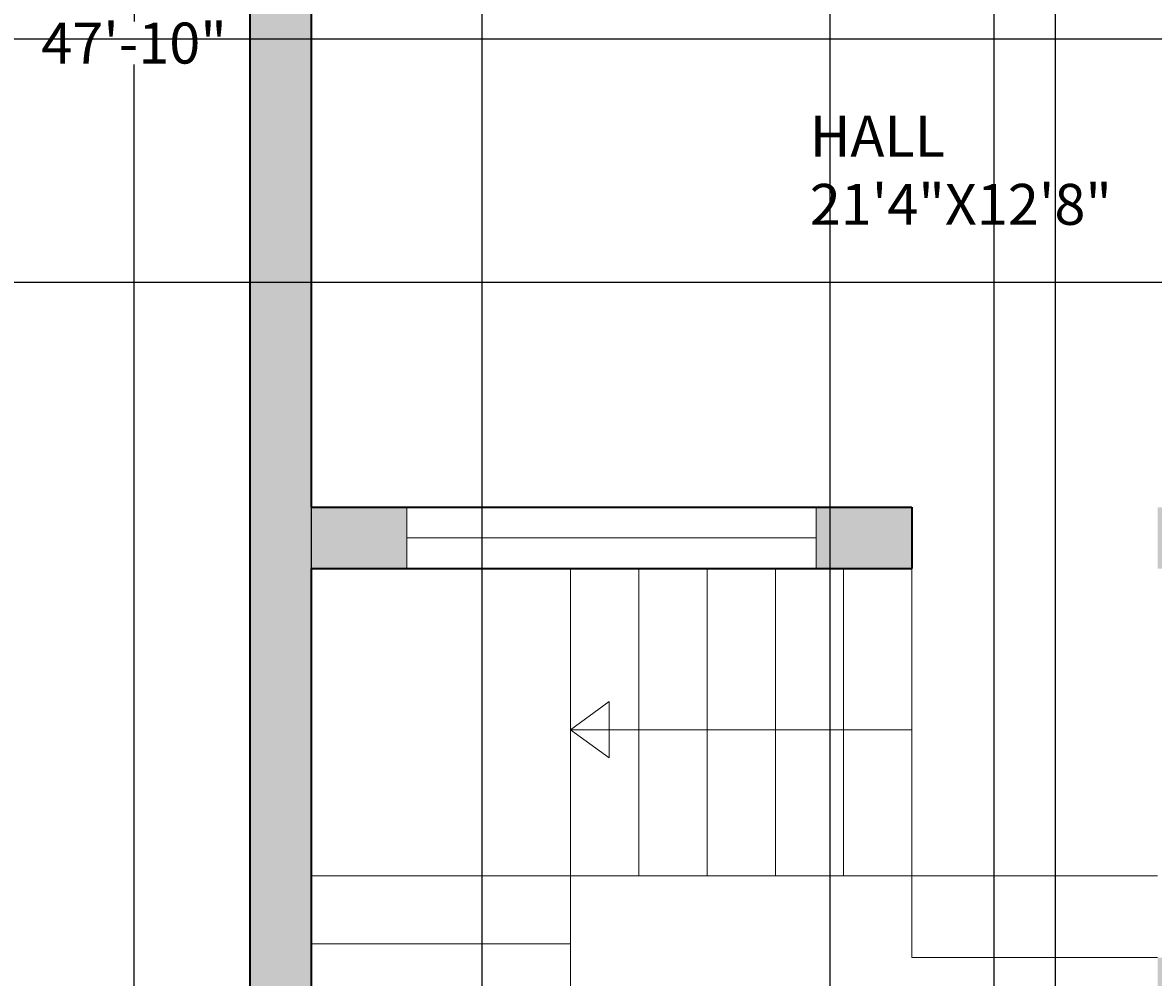
# Model space of a CAD drawing. Units: inches. Extents: x 37 to 706, y -568 to 110.
# Tile 15 of 24: x 361 to 526, y -373 to -233. Entities that reach past the tile are written whole.
import ezdxf

# ---------------------------------------------------------------- set-up
doc = ezdxf.new("R2010")
doc.units = ezdxf.units.IN
doc.header["$MEASUREMENT"] = 0
for name, color, linetype, lineweight in [('A-ANNO-DIMS', 2, 'Continuous', 18), ('A-AREA-IDEN', 7, 'Continuous', 18), ('A-FLOR-STRS', 7, 'Continuous', 18), ('A-GLAZ', 4, 'Continuous', 18), ('A-WALL', 7, 'Continuous', 35), ('A-WALL-PATT', 252, 'Continuous', 13)]:
    doc.layers.add(name, color=color, linetype=linetype, lineweight=lineweight)
doc.styles.get("Standard").update_dxf_attribs({"font": 'arial.ttf'})
doc.dimstyles.get("Standard").update_dxf_attribs({"dimtxt": 0.18, "dimasz": 0.18, "dimexe": 0.18, "dimexo": 0.0625, "dimgap": 0.09, "dimtad": 0, "dimtih": 1, "dimtoh": 1, "dimdec": 0, "dimzin": 0, "dimdsep": 46, "dimlunit": 3, "dimtxsty": 'Standard', "dimcen": 0.09, "dimadec": 0, "dimazin": 0, "dimtfac": 1, "dimtdec": 0, "dimtofl": 0, "dimtmove": 0, "dimatfit": 3, "dimfxl": 1, "dimtolj": 1, "dimtzin": 0, "dimarcsym": 0})

# ---------------------------------------------------------------- blocks, each defined once
blk = doc.blocks.new('*D5')
at = {"layer": 'A-ANNO-DIMS', "color": 0, "lineweight": -2, "transparency": 16777216}
for p, q in [((393.9, 51.29), (376.84, 51.29)), ((377.02, 51.11), (377.02, -232.56)), ((377.02, -522.53), (377.02, -238.86)), ((393.9, -522.71), (376.84, -522.71))]:
    blk.add_line(p, q, dxfattribs=at)
at = {"layer": 'A-ANNO-DIMS', "color": 0, "transparency": 16777216}
for points in [[(376.99, 51.11), (377.05, 51.11), (377.02, 51.29)], [(376.99, -522.53), (377.05, -522.53), (377.02, -522.71)]]:
    blk.add_solid(points, dxfattribs=at)
at = {"layer": 'Defpoints', "color": 0, "transparency": 16777216}
for p in [(393.96, 51.29), (377.02, -522.71), (393.96, -522.71)]:
    blk.add_point(p, dxfattribs=at)
at = {"layer": 'A-ANNO-DIMS', "color": 0, "transparency": 16777216, "insert": (377.02, -235.71), "char_height": 6, "attachment_point": 5}
blk.add_mtext('\\A1;47\'-10"', dxfattribs=at)
blk = doc.blocks.new('WIN-60')
for p, q in [((60, 9), (0, 9)), ((0, 9), (0, 0)), ((60, 0), (60, 9)), ((60, 4.5), (0, 4.5)), ((0, 0), (60, 0))]:
    blk.add_line(p, q)
blk = doc.blocks.new('*D50')
at = {"layer": 'A-ANNO-DIMS', "color": 0, "lineweight": -2, "transparency": 16777216}
for p, q in [((340.88, -235.09), (705.89, -235.09)), ((705.71, -235.27), (705.71, -252.74)), ((705.71, -270.57), (705.71, -253.1)), ((340.88, -270.75), (705.89, -270.75))]:
    blk.add_line(p, q, dxfattribs=at)
at = {"layer": 'A-ANNO-DIMS', "color": 0, "transparency": 16777216}
for points in [[(705.68, -235.27), (705.74, -235.27), (705.71, -235.09)], [(705.68, -270.57), (705.74, -270.57), (705.71, -270.75)]]:
    blk.add_solid(points, dxfattribs=at)
at = {"layer": 'Defpoints', "color": 0, "transparency": 16777216}
for p in [(340.81, -235.09), (340.81, -270.75), (705.71, -270.75)]:
    blk.add_point(p, dxfattribs=at)
at = {"layer": 'A-ANNO-DIMS', "color": 0, "transparency": 16777216, "insert": (705.71, -252.92), "char_height": 0.18, "attachment_point": 5}
blk.add_mtext('\\A1;2\'-11 1/2"', dxfattribs=at)
blk = doc.blocks.new('*D53')
at = {"layer": 'A-ANNO-DIMS', "color": 0, "lineweight": -2, "transparency": 16777216}
for p, q in [((511.96, -151.77), (511.96, -567.64)), ((537.96, -151.77), (537.96, -567.64)), ((512.14, -567.46), (524.63, -567.46)), ((537.78, -567.46), (525.29, -567.46))]:
    blk.add_line(p, q, dxfattribs=at)
at = {"layer": 'A-ANNO-DIMS', "color": 0, "transparency": 16777216}
for points in [[(512.14, -567.43), (512.14, -567.49), (511.96, -567.46)], [(537.78, -567.43), (537.78, -567.49), (537.96, -567.46)]]:
    blk.add_solid(points, dxfattribs=at)
at = {"layer": 'Defpoints', "color": 0, "transparency": 16777216}
for p in [(511.96, -151.71), (537.96, -151.71), (537.96, -567.46)]:
    blk.add_point(p, dxfattribs=at)
at = {"layer": 'A-ANNO-DIMS', "color": 0, "transparency": 16777216, "insert": (524.96, -567.46), "char_height": 0.18, "attachment_point": 5}
blk.add_mtext('\\A1;2\'-2"', dxfattribs=at)
blk = doc.blocks.new('*D56')
at = {"layer": 'A-ANNO-DIMS', "color": 0, "lineweight": -2, "transparency": 16777216}
for p, q in [((402.96, -142.77), (402.96, -567.64)), ((427.97, -142.77), (427.97, -567.64)), ((403.14, -567.46), (415.13, -567.46)), ((427.79, -567.46), (415.79, -567.46))]:
    blk.add_line(p, q, dxfattribs=at)
at = {"layer": 'A-ANNO-DIMS', "color": 0, "transparency": 16777216}
for points in [[(403.14, -567.43), (403.14, -567.49), (402.96, -567.46)], [(427.79, -567.43), (427.79, -567.49), (427.97, -567.46)]]:
    blk.add_solid(points, dxfattribs=at)
at = {"layer": 'Defpoints', "color": 0, "transparency": 16777216}
for p in [(402.96, -142.71), (427.97, -142.71), (427.97, -567.46)]:
    blk.add_point(p, dxfattribs=at)
at = {"layer": 'A-ANNO-DIMS', "color": 0, "transparency": 16777216, "insert": (415.46, -567.46), "char_height": 0.18, "attachment_point": 5}
blk.add_mtext('\\A1;2\'-1"', dxfattribs=at)
blk = doc.blocks.new('*D63')
at = {"layer": 'A-ANNO-DIMS', "color": 0, "lineweight": -2, "transparency": 16777216}
for p, q in [((478.96, -142.77), (478.96, -567.64)), ((502.96, -151.77), (502.96, -567.64)), ((479.14, -567.46), (490.63, -567.46)), ((502.78, -567.46), (491.29, -567.46))]:
    blk.add_line(p, q, dxfattribs=at)
at = {"layer": 'A-ANNO-DIMS', "color": 0, "transparency": 16777216}
for points in [[(479.14, -567.43), (479.14, -567.49), (478.96, -567.46)], [(502.78, -567.43), (502.78, -567.49), (502.96, -567.46)]]:
    blk.add_solid(points, dxfattribs=at)
at = {"layer": 'Defpoints', "color": 0, "transparency": 16777216}
for p in [(478.96, -142.71), (502.96, -151.71), (502.96, -567.46)]:
    blk.add_point(p, dxfattribs=at)
at = {"layer": 'A-ANNO-DIMS', "color": 0, "transparency": 16777216, "insert": (490.96, -567.46), "char_height": 0.18, "attachment_point": 5}
blk.add_mtext('\\A1;2\'-0"', dxfattribs=at)

msp = doc.modelspace()

# ---------------------------------------------------------------- hatches: boundary and pattern name
at = {"layer": 'A-WALL-PATT'}
h = msp.add_hatch(color=256, dxfattribs=at)
h.dxf.hatch_style = 1
h.paths.add_polyline_path([(220.96, -351.71), (211.96, -351.71), (211.96, -513.71), (254.96, -513.71), (254.96, -504.71), (220.96, -504.71)], flags=17)
h.paths.add_polyline_path([(220.96, -294.71), (211.96, -294.71), (211.96, -303.71), (220.96, -303.71)], flags=17)
h.paths.add_polyline_path([(175.96, -294.71), (155.87, -294.71), (155.87, -303.71), (155.96, -303.71), (175.96, -303.71)], flags=17)
h.paths.add_polyline_path([(220.96, -16.71), (211.96, -16.71), (211.96, -142.71), (220.96, -142.71)], flags=17)
h.paths.add_polyline_path([(357.96, 51.29), (78.96, 51.29), (78.96, -513.71), (87.96, -513.71), (87.96, -303.71), (95.87, -303.71), (95.87, -294.71), (87.96, -294.71), (87.96, -142.71), (187.96, -142.71), (187.96, -133.71), (87.96, -133.71), (87.96, -25.71), (106.96, -25.71), (106.96, -16.71), (87.96, -16.71), (87.96, 42.29), (348.96, 42.29), (348.96, 17.13), (348.96, -133.71), (246.96, -133.71), (246.96, -142.71), (348.96, -142.71), (348.96, -294.71), (251.96, -294.71), (251.96, -303.71), (348.96, -303.71), (348.96, -351.71), (260.96, -351.71), (260.96, -329.71), (251.96, -329.71), (251.96, -360.71), (327.45, -360.71), (348.96, -360.71), (348.96, -504.71), (314.96, -504.71), (314.96, -513.71), (357.96, -513.71)])
h.paths.add_polyline_path([(416.96, -303.71), (402.96, -303.71), (402.96, -151.71), (478.96, -151.71), (478.96, -142.71), (402.96, -142.71), (402.96, -22.71), (409.96, -22.71), (409.96, -13.71), (402.96, -13.71), (402.96, 42.29), (663.96, 42.29), (663.96, -303.71), (566.96, -303.71), (566.96, -312.71), (663.96, -312.71), (663.96, -360.71), (575.96, -360.71), (575.96, -338.71), (566.96, -338.71), (566.96, -360.71), (566.96, -369.71), (642.45, -369.71), (663.96, -369.71), (663.96, -513.71), (629.96, -513.71), (629.96, -522.71), (672.96, -522.71), (672.96, 51.29), (393.96, 51.29), (393.96, -522.71), (402.96, -522.71), (402.96, -312.71), (416.96, -312.71)])
h.paths.add_polyline_path([(490.96, -303.71), (476.96, -303.71), (476.96, -312.71), (490.96, -312.71)], flags=17)
h.paths.add_polyline_path([(535.96, -303.71), (526.96, -303.71), (526.96, -312.71), (535.96, -312.71)], flags=17)
h.paths.add_polyline_path([(535.96, -369.71), (526.96, -369.71), (526.96, -522.71), (569.96, -522.71), (569.96, -513.71), (535.96, -513.71)], flags=17)
h.paths.add_polyline_path([(511.96, -13.71), (502.96, -13.71), (502.96, -151.71), (511.96, -151.71)], flags=17)
h.paths.add_polyline_path([(651.54, -142.71), (651.54, -120.18), (642.54, -120.18), (642.54, -142.71), (550.54, -142.71), (550.54, -120.71), (541.54, -120.71), (541.54, -142.71), (537.96, -142.71), (537.96, -151.71), (651.54, -151.71)], flags=17)
h.paths.add_polyline_path([(651.54, -85.71), (541.54, -85.71), (541.54, -94.71), (651.54, -94.71)], flags=17)
h.paths.add_polyline_path([(476.96, -13.71), (469.96, -13.71), (469.96, -22.71), (476.96, -22.71)], flags=17)
h.paths.add_polyline_path([(185.96, -16.71), (166.96, -16.71), (166.96, -25.71), (185.96, -25.71)], flags=17)
h.paths.add_polyline_path([(168.91, -414.72), (214.62, -414.72), (214.62, -392.33), (168.91, -392.33)], flags=25)

# ---------------------------------------------------------------- linework, layer by layer
at = {"layer": 'A-FLOR-STRS'}
for p, q in [((440.96, -312.71), (440.96, -357.71)), ((450.96, -312.71), (450.96, -357.71)), ((460.96, -312.71), (460.96, -357.71)), ((470.96, -312.71), (470.96, -357.71)), ((470.96, -312.71), (470.96, -357.71)), ((480.96, -312.71), (480.96, -357.71)), ((490.96, -312.71), (490.96, -369.71)), ((440.96, -336.31), (446.61, -332.16)), ((446.61, -332.16), (446.61, -336.31)), ((490.96, -336.31), (440.96, -336.31)), ((440.96, -336.31), (446.61, -340.45)), ((446.61, -340.45), (446.61, -336.31)), ((490.96, -357.71), (402.96, -357.71)), ((440.96, -357.71), (440.96, -467.71)), ((490.96, -357.71), (526.96, -357.71)), ((440.96, -367.71), (402.96, -367.71)), ((490.96, -369.71), (526.96, -369.71))]:
    msp.add_line(p, q, dxfattribs=at)
at = {"layer": 'A-WALL'}
for p, q in [((393.96, 51.29), (393.96, -522.71)), ((402.96, -151.71), (402.96, -303.71)), ((402.96, -303.71), (490.96, -303.71)), ((490.96, -303.71), (490.96, -312.71)), ((402.96, -312.71), (490.96, -312.71)), ((402.96, -312.71), (402.96, -522.71))]:
    msp.add_line(p, q, dxfattribs=at)

# ---------------------------------------------------------------- block references
at = {"layer": 'A-GLAZ'}
msp.add_blockref('WIN-60', (416.96, -312.71), dxfattribs=at)

# ---------------------------------------------------------------- texts
at = {"layer": 'A-AREA-IDEN', "insert": (476, -246.34), "char_height": 6, "attachment_point": 1}
msp.add_mtext('HALL\\P21\'4"X12\'8"', dxfattribs=at)

# ---------------------------------------------------------------- dimensions: what is measured, and where the dimension line sits
at = {"layer": 'A-ANNO-DIMS'}
for base, p1, p2, override, picture, middle in [((377.02, -522.71), (393.96, 51.29), (393.96, -522.71), {"dimtxt": 6, "dimclrd": 0, "dimclre": 0, "dimclrt": 0}, '*D5', (377.02, -235.71)), ((705.71, -270.75), (340.81, -235.09), (340.81, -270.75), {"dimdec": 1, "dimlfac": 1, "dimrnd": 0, "dimzin": 1, "dimdsep": 46, "dimlunit": 4, "dimfrac": 2}, '*D50', (705.71, -252.92))]:
    dim = msp.add_linear_dim(base=base, p1=p1, p2=p2, angle=90, dimstyle='Standard', override=override, dxfattribs=at)
    dim.commit()
    dim.dimension.update_dxf_attribs({"geometry": picture, "text_midpoint": middle})
for base, p1, p2, picture, middle in [((427.97, -567.46), (402.96, -142.71), (427.97, -142.71), '*D56', (415.46, -567.46)), ((502.96, -567.46), (478.96, -142.71), (502.96, -151.71), '*D63', (490.96, -567.46)), ((537.96, -567.46), (511.96, -151.71), (537.96, -151.71), '*D53', (524.96, -567.46))]:
    dim = msp.add_linear_dim(base=base, p1=p1, p2=p2, dimstyle='Standard', override={"dimdec": 1, "dimlfac": 1, "dimrnd": 0, "dimzin": 1, "dimdsep": 46, "dimlunit": 4, "dimfrac": 2}, dxfattribs=at)
    dim.commit()
    dim.dimension.update_dxf_attribs({"geometry": picture, "text_midpoint": middle})

doc.saveas('drawing.dxf')
